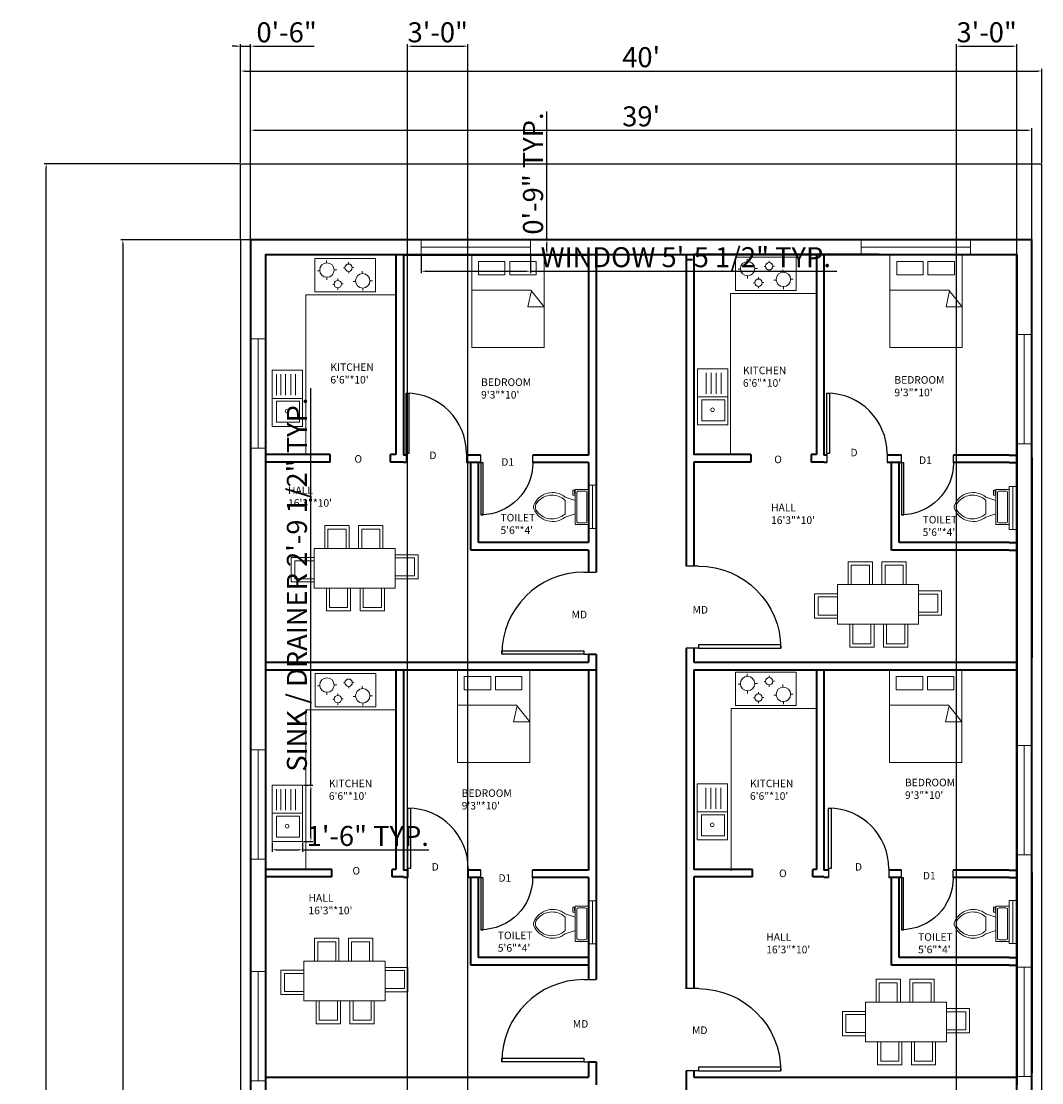
# Model space of a CAD drawing. Units: inches. Extents: x 1947 to 2903, y 1974 to 3472.
# Tile 5 of 5: x 2132 to 2743, y 2836 to 3472. Entities that reach past the tile are written whole.
import ezdxf

# ---------------------------------------------------------------- set-up
doc = ezdxf.new("R2010")
doc.units = ezdxf.units.IN
for name, color, linetype, lineweight in [('A-ANNO-DIMS', 2, 'Continuous', 18), ('A-ANNO-TEXT', 7, 'Continuous', 18), ('A-AREA-IDEN', 7, 'Continuous', 18), ('A-DOOR', 3, 'Continuous', 25), ('A-EQPM', 8, 'Continuous', 18), ('A-FLOR-CASE', 8, 'Continuous', 18), ('A-FLOR-FIXT', 9, 'Continuous', 18), ('A-FURN', 8, 'Continuous', 18), ('A-GLAZ', 4, 'Continuous', 18), ('A-GLAZ-VENT', 4, 'Continuous', 18), ('A-WALL', 7, 'Continuous', 35), ('C-PROP', 1, 'Continuous', 25)]:
    doc.layers.add(name, color=color, linetype=linetype, lineweight=lineweight)
doc.styles.get("Standard").update_dxf_attribs({"font": 'arial.ttf'})
doc.dimstyles.new('ISO-25', dxfattribs={"dimtxt": 12, "dimasz": 2.5, "dimexe": 1.25, "dimexo": 0.625, "dimtad": 1, "dimdec": 0, "dimlunit": 4, "dimtxsty": 'Standard', "dimcen": 2.5, "dimadec": 0, "dimazin": 0, "dimtfac": 1, "dimtdec": 0, "dimtmove": 0, "dimatfit": 3, "dimfxl": 1, "dimarcsym": 0})

# ---------------------------------------------------------------- blocks, each defined once
blk = doc.blocks.new('*U2')
for p, q in [((0, 0), (0, -6)), ((40, 0), (40, -6))]:
    blk.add_line(p, q)
blk.add_lwpolyline([(0, 0), (0, 40), (1.75, 40), (1.75, 0)], close=True)
blk.add_arc((0, 0), 40, 0, 90)
blk = doc.blocks.new('*U4')
for p, q in [((9.5, -6), (9.5, -2)), ((-10, -8.5), (-8, -8.5)), ((-10, -9.5), (-10, -8.5)), ((-7, -9.5), (-10, -9.5)), ((-8, -8.5), (-8, -8)), ((-7, -8), (-7, -9.5)), ((-4, -8), (-6, -14)), ((4, -8), (6, -14)), ((4, -14), (-4, -14))]:
    blk.add_line(p, q)
blk.add_lwpolyline([(10.5, -8), (10.5, 0), (-10.5, 0), (-10.5, -8)], close=True)
for points in [[(-9.5, -2), (-9.5, -6)], [(8.5, -1), (-8.5, -1)], [(-8.5, -7), (8.5, -7)]]:
    blk.add_lwpolyline(points)
for centre, radius, start, end in [((-8.62, -1.88), 0.884, 81.8699, 188.1301), ((-8.62, -6.12), 0.884, 171.8699, 278.1301), ((8.62, -1.88), 0.884, 351.8699, 98.1301), ((8.62, -6.12), 0.884, 261.8699, 8.1301), ((3.52, -21.58), 12.17, 141.46911, 247.97143), ((4.2, -21.82), 11.33, 136.36773, 238.94682), ((-3.52, -21.58), 12.17, 292.02843, 38.53071), ((-4.2, -21.82), 11.33, 301.05301, 43.63209), ((0, -27.88), 4, 245.73182, 294.26817), ((0, -29), 4, 254.86053, 285.13947)]:
    blk.add_arc(centre, radius, start, end)
blk = doc.blocks.new('*D5')
at = {"layer": 'A-ANNO-DIMS', "color": 0, "lineweight": -2, "transparency": 16777216}
for p, q in [((2269.11, 3342.03), (2269.11, 3408.29)), ((2271.61, 3407.04), (2734.61, 3407.04)), ((2737.11, 3342.03), (2737.11, 3408.29))]:
    blk.add_line(p, q, dxfattribs=at)
at = {"layer": 'A-ANNO-DIMS', "color": 0, "lineweight": 100, "transparency": 16777216}
for points in [[(2271.61, 3407.46), (2271.61, 3406.63), (2269.11, 3407.04)], [(2734.61, 3407.46), (2734.61, 3406.63), (2737.11, 3407.04)]]:
    blk.add_solid(points, dxfattribs=at)
at = {"layer": 'Defpoints', "color": 0, "lineweight": 100, "transparency": 16777216}
for p in [(2737.11, 3407.04), (2269.11, 3341.41), (2737.11, 3341.41)]:
    blk.add_point(p, dxfattribs=at)
at = {"layer": 'A-ANNO-DIMS', "color": 0, "transparency": 16777216, "insert": (2503.11, 3413.8), "char_height": 12, "attachment_point": 5}
blk.add_mtext("39'", dxfattribs=at)
blk = doc.blocks.new('*D6')
at = {"layer": 'A-ANNO-DIMS', "color": 0, "lineweight": -2, "transparency": 16777216}
for p, q in [((2268.49, 3341.41), (2191.31, 3341.41)), ((2192.56, 3338.91), (2192.56, 2230.91)), ((2268.49, 2228.41), (2191.31, 2228.41))]:
    blk.add_line(p, q, dxfattribs=at)
at = {"layer": 'A-ANNO-DIMS', "color": 0, "lineweight": 100, "transparency": 16777216}
for points in [[(2192.15, 3338.91), (2192.98, 3338.91), (2192.56, 3341.41)], [(2192.15, 2230.91), (2192.98, 2230.91), (2192.56, 2228.41)]]:
    blk.add_solid(points, dxfattribs=at)
at = {"layer": 'Defpoints', "color": 0, "lineweight": 100, "transparency": 16777216}
for p in [(2269.11, 3341.41), (2192.56, 2228.41), (2269.11, 2228.41)]:
    blk.add_point(p, dxfattribs=at)
at = {"layer": 'A-ANNO-DIMS', "color": 0, "transparency": 16777216, "insert": (2185.81, 2784.91), "char_height": 12, "attachment_point": 5, "rotation": 90}
blk.add_mtext('92\'-9"', dxfattribs=at)
blk = doc.blocks.new('*D7')
at = {"layer": 'A-ANNO-DIMS', "color": 0, "lineweight": -2, "transparency": 16777216}
for p, q in [((2263.11, 3387.59), (2263.11, 3443.75)), ((2265.61, 3442.5), (2740.61, 3442.5)), ((2743.11, 3387.59), (2743.11, 3443.75))]:
    blk.add_line(p, q, dxfattribs=at)
at = {"layer": 'A-ANNO-DIMS', "color": 0, "lineweight": 100, "transparency": 16777216}
for points in [[(2265.61, 3442.92), (2265.61, 3442.09), (2263.11, 3442.5)], [(2740.61, 3442.92), (2740.61, 3442.09), (2743.11, 3442.5)]]:
    blk.add_solid(points, dxfattribs=at)
at = {"layer": 'Defpoints', "color": 0, "lineweight": 100, "transparency": 16777216}
for p in [(2743.11, 3442.5), (2263.11, 3386.97), (2743.11, 3386.97)]:
    blk.add_point(p, dxfattribs=at)
at = {"layer": 'A-ANNO-DIMS', "color": 0, "transparency": 16777216, "insert": (2503.11, 3449.26), "char_height": 12, "attachment_point": 5}
blk.add_mtext("40'", dxfattribs=at)
blk = doc.blocks.new('*D8')
at = {"layer": 'A-ANNO-DIMS', "color": 0, "lineweight": -2, "transparency": 16777216}
for p, q in [((2262.49, 3386.97), (2145.36, 3386.97)), ((2146.61, 2187.91), (2146.61, 3384.47)), ((2262.49, 2185.41), (2145.36, 2185.41))]:
    blk.add_line(p, q, dxfattribs=at)
at = {"layer": 'A-ANNO-DIMS', "color": 0, "lineweight": 100, "transparency": 16777216}
for points in [[(2146.19, 3384.47), (2147.03, 3384.47), (2146.61, 3386.97)], [(2146.19, 2187.91), (2147.03, 2187.91), (2146.61, 2185.41)]]:
    blk.add_solid(points, dxfattribs=at)
at = {"layer": 'Defpoints', "color": 0, "lineweight": 100, "transparency": 16777216}
for p in [(2146.61, 3386.97), (2263.11, 3386.97), (2263.11, 2185.41)]:
    blk.add_point(p, dxfattribs=at)
at = {"layer": 'A-ANNO-DIMS', "color": 0, "transparency": 16777216, "insert": (2139.86, 2786.19), "char_height": 12, "attachment_point": 5, "rotation": 90}
blk.add_mtext('100\'-2"', dxfattribs=at)
blk = doc.blocks.new('BED-TWO-PILLOWS')
for p, q in [((0, 34.29), (35.37, 34.29)), ((33.59, 24.29), (35.7, 33.87)), ((35.37, 34.29), (43.32, 24.29)), ((43.32, 24.29), (33.59, 24.29))]:
    blk.add_line(p, q)
for points in [[(0, 55.57), (43.32, 55.57), (43.32, 0), (0, 0)], [(4.07, 51.54), (19.88, 51.54), (19.88, 43.48), (4.07, 43.48)], [(22.78, 51.54), (38.59, 51.54), (38.59, 43.48), (22.78, 43.48)]]:
    blk.add_lwpolyline(points, close=True)
blk = doc.blocks.new('DINING-SET-6')
for p, q in [((20.16, 37.5), (20.16, 51.24)), ((20.16, 51.24), (34.7, 51.24)), ((34.7, 51.24), (34.7, 37.5)), ((40.4, 37.5), (40.4, 51.24)), ((40.4, 51.24), (54.94, 51.24)), ((54.94, 51.24), (54.94, 37.5)), ((13.74, 31.99), (0, 31.99)), ((0, 31.99), (0, 17.45)), ((62.33, 33.71), (76.07, 33.71)), ((76.07, 33.71), (76.07, 19.17)), ((76.07, 19.17), (62.33, 19.17)), ((0, 17.45), (13.74, 17.45)), ((21.08, 13.74), (21.08, 0)), ((35.62, 0), (35.62, 13.74)), ((41.32, 13.74), (41.32, 0)), ((55.86, 0), (55.86, 13.74)), ((21.08, 0), (35.62, 0)), ((41.32, 0), (55.86, 0))]:
    blk.add_line(p, q)
for points in [[(22.02, 37.5), (32.87, 37.5), (32.87, 49.12), (22.02, 49.12)], [(42.26, 37.5), (53.11, 37.5), (53.11, 49.12), (42.26, 49.12)], [(13.74, 13.74), (62.33, 13.74), (62.33, 37.5), (13.74, 37.5)], [(62.33, 31.85), (62.33, 21), (73.95, 21), (73.95, 31.85)], [(13.74, 30.13), (13.74, 19.28), (2.12, 19.28), (2.12, 30.13)], [(22.94, 13.74), (33.79, 13.74), (33.79, 2.12), (22.94, 2.12)], [(43.18, 13.74), (54.03, 13.74), (54.03, 2.12), (43.18, 2.12)]]:
    blk.add_lwpolyline(points, close=True)
blk = doc.blocks.new('COOKTOP-4-BURNER')
for p, q in [((6.9, 17.32), (6.9, 18.83)), ((11.47, 13.09), (13.05, 13.09)), ((17.95, 14.27), (17.07, 14.27)), ((20.11, 16.62), (20.11, 17.76)), ((22.35, 14.5), (23.33, 14.5)), ((2.85, 12.63), (1.48, 12.63)), ((7.15, 8.69), (7.15, 7.15)), ((13.68, 6.8), (13.68, 7.94)), ((20.18, 12.22), (20.18, 11.07)), ((28.35, 10.88), (28.35, 12.39)), ((32.92, 6.64), (34.51, 6.64)), ((11.52, 4.44), (10.65, 4.44)), ((13.75, 2.39), (13.75, 1.25)), ((15.92, 4.68), (16.91, 4.68)), ((24.3, 6.18), (22.93, 6.18)), ((28.6, 2.24), (28.6, 0.7))]:
    blk.add_line(p, q)
blk.add_lwpolyline([(0, 0), (36.35, 0), (36.35, 19.93), (0, 19.93)], close=True)
for centre, radius in [((7.15, 13.01), 4.32), ((20.14, 14.42), 2.2), ((13.72, 4.6), 2.2), ((28.6, 6.56), 4.32)]:
    blk.add_circle(centre, radius)
blk = doc.blocks.new('SINK-DRAINER-5')
for p, q in [((2.58, 18.66), (2.58, 31.31)), ((5.19, 18.66), (5.19, 31.31)), ((8.1, 18.66), (8.1, 31.31)), ((11.22, 18.66), (11.22, 31.31)), ((14.13, 18.66), (14.13, 31.31)), ((0, 16.81), (18.23, 16.81))]:
    blk.add_line(p, q)
for points in [[(0, 0), (18.23, 0), (18.23, 33.61), (0, 33.61)], [(2.68, 15.14), (16.44, 15.14), (16.44, 2.49), (2.68, 2.49)]]:
    blk.add_lwpolyline(points, close=True)
blk.add_circle((9.01, 9.12), 1.11)
blk = doc.blocks.new('SINK-DRAINER-4')
for p, q in [((5.19, 18.66), (5.19, 31.31)), ((8.1, 18.66), (8.1, 31.31)), ((11.22, 18.66), (11.22, 31.31)), ((14.13, 18.66), (14.13, 31.31)), ((0, 16.81), (18.23, 16.81))]:
    blk.add_line(p, q)
for points in [[(0, 0), (18.23, 0), (18.23, 33.61), (0, 33.61)], [(2.68, 15.14), (16.44, 15.14), (16.44, 2.49), (2.68, 2.49)]]:
    blk.add_lwpolyline(points, close=True)
blk.add_circle((9.01, 9.12), 1.11)
blk = doc.blocks.new('WINDOW-EXTERIOR')
blk.add_line((0, 4.5), (65.51, 4.5))
blk.add_lwpolyline([(0, 0), (65.51, 0), (65.51, 9), (0, 9)], close=True)
blk = doc.blocks.new('VENT-TOILET')
blk.add_line((2.25, 0), (2.25, 25.89))
blk.add_lwpolyline([(0, 25.89), (4.5, 25.89), (4.5, 0), (0, 0)], close=True)
blk = doc.blocks.new('COOKTOP-4-BURNER-B')
for p, q in [((11.47, 13.09), (13.05, 13.09)), ((17.95, 14.27), (17.07, 14.27)), ((22.35, 14.5), (23.33, 14.5)), ((2.85, 12.63), (1.48, 12.63)), ((7.15, 8.69), (7.15, 7.15)), ((13.68, 6.8), (13.68, 7.94)), ((20.18, 12.22), (20.18, 11.07)), ((28.35, 10.88), (28.35, 12.39)), ((32.92, 6.64), (34.51, 6.64)), ((11.52, 4.44), (10.65, 4.44)), ((13.75, 2.4), (13.75, 1.25)), ((15.92, 4.68), (16.91, 4.68)), ((24.3, 6.18), (22.93, 6.18)), ((28.6, 2.24), (28.6, 0.71))]:
    blk.add_line(p, q)
blk.add_lwpolyline([(0, 0), (36.35, 0), (36.35, 19.93), (0, 19.93)], close=True)
for centre, radius in [((7.15, 13.01), 4.32), ((20.14, 14.42), 2.2), ((13.72, 4.6), 2.2), ((28.6, 6.56), 4.32)]:
    blk.add_circle(centre, radius)
blk = doc.blocks.new('*D17')
at = {"layer": 'A-ANNO-DIMS', "color": 0, "lineweight": -2, "transparency": 16777216}
for p, q in [((2371.28, 3331.78), (2371.28, 3321.33)), ((2436.79, 3331.78), (2436.79, 3321.33)), ((2373.78, 3322.58), (2434.29, 3322.58)), ((2436.79, 3322.58), (2620.35, 3322.58))]:
    blk.add_line(p, q, dxfattribs=at)
at = {"layer": 'A-ANNO-DIMS', "color": 0, "lineweight": 100, "transparency": 16777216}
for points in [[(2373.78, 3323), (2373.78, 3322.16), (2371.28, 3322.58)], [(2434.29, 3323), (2434.29, 3322.16), (2436.79, 3322.58)]]:
    blk.add_solid(points, dxfattribs=at)
at = {"layer": 'Defpoints', "color": 0, "lineweight": 100, "transparency": 16777216}
for p in [(2371.28, 3332.41), (2436.79, 3332.41), (2436.79, 3322.58)]:
    blk.add_point(p, dxfattribs=at)
at = {"layer": 'A-ANNO-DIMS', "color": 0, "transparency": 16777216, "insert": (2529.82, 3329.41), "char_height": 12, "attachment_point": 5}
blk.add_mtext('WINDOW 5\'-5 1/2" TYP.', dxfattribs=at)
blk = doc.blocks.new('*D18')
at = {"layer": 'A-ANNO-DIMS', "color": 0, "lineweight": -2, "transparency": 16777216}
for p, q in [((2446.62, 3341.41), (2446.62, 3418.3)), ((2437.42, 3341.41), (2447.87, 3341.41)), ((2446.62, 3334.91), (2446.62, 3338.91)), ((2437.42, 3332.41), (2447.87, 3332.41))]:
    blk.add_line(p, q, dxfattribs=at)
at = {"layer": 'A-ANNO-DIMS', "color": 0, "lineweight": 100, "transparency": 16777216}
for points in [[(2446.2, 3338.91), (2447.03, 3338.91), (2446.62, 3341.41)], [(2446.2, 3334.91), (2447.03, 3334.91), (2446.62, 3332.41)]]:
    blk.add_solid(points, dxfattribs=at)
at = {"layer": 'Defpoints', "color": 0, "lineweight": 100, "transparency": 16777216}
for p in [(2436.79, 3341.41), (2446.62, 3341.41), (2436.79, 3332.41)]:
    blk.add_point(p, dxfattribs=at)
at = {"layer": 'A-ANNO-DIMS', "color": 0, "transparency": 16777216, "insert": (2439.86, 3381.1), "char_height": 12, "attachment_point": 5, "rotation": 90}
blk.add_mtext('0\'-9" TYP.', dxfattribs=at)
blk = doc.blocks.new('*D27')
at = {"layer": 'A-ANNO-DIMS', "color": 0, "lineweight": -2, "transparency": 16777216}
for p, q in [((2305.22, 3014.51), (2305.22, 3252.52)), ((2300.8, 3014.51), (2306.47, 3014.51)), ((2305.22, 2983.4), (2305.22, 3012.01)), ((2300.8, 2980.9), (2306.47, 2980.9))]:
    blk.add_line(p, q, dxfattribs=at)
at = {"layer": 'A-ANNO-DIMS', "color": 0, "lineweight": 100, "transparency": 16777216}
for points in [[(2304.8, 3012.01), (2305.64, 3012.01), (2305.22, 3014.51)], [(2304.8, 2983.4), (2305.64, 2983.4), (2305.22, 2980.9)]]:
    blk.add_solid(points, dxfattribs=at)
at = {"layer": 'Defpoints', "color": 0, "lineweight": 100, "transparency": 16777216}
for p in [(2300.18, 3014.51), (2305.22, 3014.51), (2300.18, 2980.9)]:
    blk.add_point(p, dxfattribs=at)
at = {"layer": 'A-ANNO-DIMS', "color": 0, "transparency": 16777216, "insert": (2298.39, 3134.77), "char_height": 12, "attachment_point": 5, "rotation": 90}
blk.add_mtext('SINK / DRAINER 2\'-9 1/2" TYP.', dxfattribs=at)
blk = doc.blocks.new('*D28')
at = {"layer": 'A-ANNO-DIMS', "color": 0, "lineweight": -2, "transparency": 16777216}
for p, q in [((2281.94, 2980.27), (2281.94, 2974.61)), ((2300.18, 2980.27), (2300.18, 2974.61)), ((2284.44, 2975.86), (2297.68, 2975.86)), ((2300.18, 2975.86), (2375.94, 2975.86))]:
    blk.add_line(p, q, dxfattribs=at)
at = {"layer": 'A-ANNO-DIMS', "color": 0, "lineweight": 100, "transparency": 16777216}
for points in [[(2284.44, 2976.27), (2284.44, 2975.44), (2281.94, 2975.86)], [(2297.68, 2976.27), (2297.68, 2975.44), (2300.18, 2975.86)]]:
    blk.add_solid(points, dxfattribs=at)
at = {"layer": 'Defpoints', "color": 0, "lineweight": 100, "transparency": 16777216}
for p in [(2281.94, 2980.9), (2300.18, 2980.9), (2300.18, 2975.86)]:
    blk.add_point(p, dxfattribs=at)
at = {"layer": 'A-ANNO-DIMS', "color": 0, "transparency": 16777216, "insert": (2339.31, 2982.61), "char_height": 12, "attachment_point": 5}
blk.add_mtext('1\'-6" TYP.', dxfattribs=at)
blk = doc.blocks.new('*D36')
at = {"layer": 'A-ANNO-DIMS', "color": 0, "lineweight": -2, "transparency": 16777216}
for p, q in [((2692.11, 2238.03), (2692.11, 3458.67)), ((2694.61, 3457.42), (2725.61, 3457.42)), ((2728.11, 2238.03), (2728.11, 3458.67))]:
    blk.add_line(p, q, dxfattribs=at)
at = {"layer": 'A-ANNO-DIMS', "color": 0, "lineweight": 100, "transparency": 16777216}
for points in [[(2694.61, 3457.83), (2694.61, 3457), (2692.11, 3457.42)], [(2725.61, 3457.83), (2725.61, 3457), (2728.11, 3457.42)]]:
    blk.add_solid(points, dxfattribs=at)
at = {"layer": 'Defpoints', "color": 0, "lineweight": 100, "transparency": 16777216}
for p in [(2728.11, 3457.42), (2692.11, 2237.41), (2728.11, 2237.41)]:
    blk.add_point(p, dxfattribs=at)
at = {"layer": 'A-ANNO-DIMS', "color": 0, "transparency": 16777216, "insert": (2710.11, 3464.17), "char_height": 12, "attachment_point": 5}
blk.add_mtext('3\'-0"', dxfattribs=at)
blk = doc.blocks.new('*D40')
at = {"layer": 'A-ANNO-DIMS', "color": 0, "lineweight": -2, "transparency": 16777216}
for p, q in [((2363.18, 2467.02), (2363.18, 3458.67)), ((2365.68, 3457.42), (2396.82, 3457.42)), ((2399.32, 2467.02), (2399.32, 3458.67))]:
    blk.add_line(p, q, dxfattribs=at)
at = {"layer": 'A-ANNO-DIMS', "color": 0, "lineweight": 100, "transparency": 16777216}
for points in [[(2365.68, 3457.83), (2365.68, 3457), (2363.18, 3457.42)], [(2396.82, 3457.83), (2396.82, 3457), (2399.32, 3457.42)]]:
    blk.add_solid(points, dxfattribs=at)
at = {"layer": 'Defpoints', "color": 0, "lineweight": 100, "transparency": 16777216}
for p in [(2399.32, 3457.42), (2363.18, 2466.39), (2399.32, 2466.39)]:
    blk.add_point(p, dxfattribs=at)
at = {"layer": 'A-ANNO-DIMS', "color": 0, "transparency": 16777216, "insert": (2381.25, 3464.17), "char_height": 12, "attachment_point": 5}
blk.add_mtext('3\'-0"', dxfattribs=at)
blk = doc.blocks.new('*D43')
at = {"layer": 'A-ANNO-DIMS', "color": 0, "lineweight": -2, "transparency": 16777216}
for p, q in [((2260.61, 3457.42), (2258.11, 3457.42)), ((2263.11, 3387.59), (2263.11, 3458.67)), ((2263.11, 3457.42), (2269.11, 3457.42)), ((2269.11, 3342.03), (2269.11, 3458.67)), ((2271.61, 3457.42), (2307.26, 3457.42))]:
    blk.add_line(p, q, dxfattribs=at)
at = {"layer": 'A-ANNO-DIMS', "color": 0, "lineweight": 100, "transparency": 16777216}
for points in [[(2260.61, 3457.83), (2260.61, 3457), (2263.11, 3457.42)], [(2271.61, 3457.83), (2271.61, 3457), (2269.11, 3457.42)]]:
    blk.add_solid(points, dxfattribs=at)
at = {"layer": 'Defpoints', "color": 0, "lineweight": 100, "transparency": 16777216}
for p in [(2269.11, 3457.42), (2263.11, 3386.97), (2269.11, 3341.41)]:
    blk.add_point(p, dxfattribs=at)
at = {"layer": 'A-ANNO-DIMS', "color": 0, "transparency": 16777216, "insert": (2290.68, 3464.17), "char_height": 12, "attachment_point": 5}
blk.add_mtext('0\'-6"', dxfattribs=at)

msp = doc.modelspace()

# ---------------------------------------------------------------- linework, layer by layer
at = {"layer": 'A-FLOR-CASE'}
for p, q in [((2356.11, 3332.41), (2356.11, 3308.41)), ((2302.11, 3212.73), (2302.11, 3308.41)), ((2356.11, 3308.41), (2302.11, 3308.41)), ((2556.71, 3213.57), (2556.71, 3309.24)), ((2608.11, 3309.24), (2556.71, 3309.24)), ((2278.11, 3212.73), (2302.11, 3212.73)), ((2302.11, 2964.06), (2302.11, 3059.73)), ((2356.11, 3059.73), (2302.11, 3059.73)), ((2557.05, 2963.31), (2557.05, 3060.58)), ((2608.11, 3060.58), (2557.05, 3060.58)), ((2278.11, 2964.06), (2302.11, 2964.06))]:
    msp.add_line(p, q, dxfattribs=at)
at = {"layer": 'A-WALL'}
for p, q in [((2356.11, 3332.41), (2356.11, 3212.73)), ((2360.61, 3332.41), (2360.61, 3212.41)), ((2360.61, 3332.41), (2471.61, 3332.41)), ((2471.61, 3332.41), (2471.61, 3212.41)), ((2476.11, 3332.41), (2476.11, 3207.91)), ((2530.11, 3332.6), (2530.11, 3208.1)), ((2645.61, 3332.6), (2534.61, 3332.6)), ((2534.61, 3332.6), (2534.61, 3212.6)), ((2608.11, 3332.41), (2608.11, 3212.73)), ((2612.61, 3332.41), (2612.61, 3212.41)), ((2728.11, 3332.41), (2728.11, 3207.91)), ((2316.73, 3212.73), (2278.11, 3212.73)), ((2316.73, 3208.23), (2316.73, 3212.73)), ((2356.11, 3212.73), (2352.86, 3212.73)), ((2352.86, 3208.23), (2352.86, 3212.73)), ((2362.29, 3212.41), (2360.61, 3212.41)), ((2407.08, 3212.41), (2398.43, 3212.41)), ((2471.61, 3212.41), (2438.18, 3212.41)), ((2530.11, 3212.73), (2530.11, 3212.73)), ((2568.73, 3212.73), (2534.61, 3212.73)), ((2568.73, 3212.73), (2568.73, 3208.23)), ((2608.11, 3212.73), (2604.86, 3212.73)), ((2604.86, 3212.73), (2604.86, 3208.23)), ((2614.29, 3212.41), (2612.61, 3212.41)), ((2659.08, 3212.41), (2650.43, 3212.41)), ((2723.61, 3212.41), (2690.18, 3212.41)), ((2723.61, 3212.41), (2728.11, 3212.41)), ((2278.11, 3208.23), (2278.11, 3088.23)), ((2316.73, 3208.23), (2278.11, 3208.23)), ((2360.61, 3208.23), (2352.86, 3208.23)), ((2362.29, 3207.91), (2360.61, 3207.91)), ((2407.08, 3207.91), (2398.43, 3207.91)), ((2401.11, 3155.41), (2401.11, 3207.91)), ((2405.61, 3159.91), (2405.61, 3207.91)), ((2471.61, 3207.91), (2438.18, 3207.91)), ((2471.61, 3207.91), (2471.61, 3159.91)), ((2476.11, 3207.91), (2476.11, 3142.22)), ((2530.11, 3208.23), (2530.11, 3208.23)), ((2530.11, 3208.1), (2530.11, 3145.81)), ((2568.73, 3208.23), (2534.61, 3208.23)), ((2534.61, 3208.23), (2534.61, 3145.81)), ((2612.61, 3208.23), (2604.86, 3208.23)), ((2614.29, 3207.91), (2612.61, 3207.91)), ((2659.08, 3207.91), (2650.43, 3207.91)), ((2653.11, 3155.41), (2653.11, 3207.91)), ((2657.61, 3159.91), (2657.61, 3207.91)), ((2723.61, 3207.91), (2690.18, 3207.91)), ((2723.61, 3207.91), (2728.11, 3207.91)), ((2728.11, 3208.43), (2728.11, 3088.43)), ((2728.11, 3207.91), (2728.11, 3142.22)), ((2737.11, 3210.89), (2737.11, 3090.89)), ((2471.61, 3155.41), (2401.11, 3155.41)), ((2471.61, 3159.91), (2405.61, 3159.91)), ((2471.61, 3155.41), (2471.61, 3142.22)), ((2723.61, 3155.41), (2653.11, 3155.41)), ((2723.61, 3159.91), (2657.61, 3159.91)), ((2723.61, 3159.91), (2728.11, 3159.91)), ((2723.61, 3155.41), (2728.11, 3155.41)), ((2471.61, 3093.01), (2476.11, 3093.01)), ((2471.61, 3093.01), (2471.61, 3088.23)), ((2476.11, 3093.01), (2476.11, 3083.73)), ((2530.11, 3096.61), (2530.11, 2892.64)), ((2534.61, 3096.61), (2534.61, 3088.23)), ((2728.11, 3093.01), (2728.11, 3083.73)), ((2278.11, 3088.23), (2471.61, 3088.23)), ((2534.61, 3088.23), (2723.61, 3088.23)), ((2723.61, 3088.23), (2728.11, 3088.23)), ((2278.11, 3083.73), (2476.11, 3083.73)), ((2356.11, 3083.73), (2356.11, 2964.06)), ((2360.61, 3083.73), (2360.61, 2963.73)), ((2360.61, 3083.73), (2471.61, 3083.73)), ((2471.61, 3083.73), (2471.61, 2963.73)), ((2476.11, 3083.73), (2476.11, 2959.23)), ((2534.61, 3083.73), (2728.11, 3083.73)), ((2534.61, 3083.73), (2534.61, 2964.06)), ((2608.11, 3083.73), (2608.11, 2964.06)), ((2612.61, 3083.73), (2612.61, 2963.73)), ((2612.61, 3083.73), (2723.61, 3083.73)), ((2728.11, 3083.73), (2728.11, 2959.23)), ((2317.8, 2964.06), (2278.11, 2964.06)), ((2316.73, 2964.06), (2278.11, 2964.06)), ((2278.11, 2959.56), (2278.11, 2839.56)), ((2317.8, 2959.56), (2278.11, 2959.56)), ((2317.8, 2959.56), (2317.8, 2964.06)), ((2356.11, 2964.06), (2353.94, 2964.06)), ((2353.94, 2959.56), (2353.94, 2964.06)), ((2360.61, 2959.56), (2353.94, 2959.56)), ((2363.37, 2963.73), (2360.61, 2963.73)), ((2363.37, 2959.23), (2360.61, 2959.23)), ((2406.98, 2963.73), (2399.51, 2963.73)), ((2406.98, 2959.23), (2399.51, 2959.23)), ((2401.11, 2906.73), (2401.11, 2959.23)), ((2405.61, 2911.23), (2405.61, 2959.23)), ((2471.61, 2963.73), (2438.08, 2963.73)), ((2471.61, 2959.23), (2438.08, 2959.23)), ((2471.61, 2959.23), (2471.61, 2911.23)), ((2476.11, 2959.23), (2476.11, 2898.05)), ((2530.11, 2964.06), (2530.11, 2964.06)), ((2530.11, 2959.56), (2530.11, 2959.56)), ((2569.81, 2964.06), (2534.61, 2964.06)), ((2569.81, 2959.56), (2534.61, 2959.56)), ((2534.61, 2959.56), (2534.61, 2892.64)), ((2569.81, 2959.56), (2569.81, 2964.06)), ((2608.11, 2964.06), (2605.94, 2964.06)), ((2605.94, 2959.56), (2605.94, 2964.06)), ((2612.61, 2959.56), (2605.94, 2959.56)), ((2615.37, 2963.73), (2612.61, 2963.73)), ((2615.37, 2959.23), (2612.61, 2959.23)), ((2658.98, 2963.73), (2651.51, 2963.73)), ((2658.98, 2959.23), (2651.51, 2959.23)), ((2653.11, 2906.73), (2653.11, 2959.23)), ((2657.61, 2911.23), (2657.61, 2959.23)), ((2723.61, 2963.73), (2690.08, 2963.73)), ((2723.61, 2959.23), (2690.08, 2959.23)), ((2723.61, 2963.73), (2728.11, 2963.73)), ((2723.61, 2959.23), (2728.11, 2959.23)), ((2728.11, 2959.76), (2728.11, 2839.76)), ((2728.11, 2959.23), (2728.11, 2898.05)), ((2737.11, 2962.22), (2737.11, 2842.22)), ((2471.61, 2911.23), (2405.61, 2911.23)), ((2471.61, 2911.23), (2471.61, 2898.05)), ((2723.61, 2911.23), (2657.61, 2911.23)), ((2723.61, 2911.23), (2728.11, 2911.23)), ((2471.61, 2906.73), (2401.11, 2906.73)), ((2471.61, 2906.73), (2471.61, 2898.05)), ((2723.61, 2906.73), (2653.11, 2906.73)), ((2723.61, 2906.73), (2728.11, 2906.73)), ((2471.61, 2848.84), (2471.61, 2844.06)), ((2471.61, 2848.84), (2476.11, 2848.84)), ((2471.61, 2848.84), (2471.61, 2839.56)), ((2476.11, 2848.84), (2476.11, 2839.56)), ((2476.11, 2848.84), (2476.11, 2835.06)), ((2530.11, 2843.44), (2530.11, 2643.97)), ((2534.61, 2843.44), (2534.61, 2839.56)), ((2728.11, 2848.84), (2728.11, 2835.06)), ((2728.11, 2848.84), (2728.11, 2839.56)), ((2278.11, 2839.56), (2471.61, 2839.56)), ((2278.11, 2839.56), (2471.61, 2839.56)), ((2534.61, 2839.56), (2723.61, 2839.56)), ((2534.61, 2839.56), (2723.61, 2839.56)), ((2723.61, 2839.56), (2728.11, 2839.56))]:
    msp.add_line(p, q, dxfattribs=at)
for points in [[(2269.11, 2228.41), (2737.11, 2228.41), (2737.11, 3341.41), (2269.11, 3341.41)], [(2278.11, 2237.41), (2728.11, 2237.41), (2728.11, 3332.41), (2278.11, 3332.41)]]:
    msp.add_lwpolyline(points, close=True, dxfattribs=at)
at = {"layer": 'C-PROP'}
for p, q in [((2263.11, 3341.17), (2263.11, 3386.97)), ((2263.11, 3386.97), (2743.11, 3386.97)), ((2743.11, 3341.41), (2743.11, 3386.97)), ((2263.11, 3341.41), (2263.11, 2228.41)), ((2743.11, 2228.41), (2743.11, 3341.41))]:
    msp.add_line(p, q, dxfattribs=at)

# ---------------------------------------------------------------- block references
at = {"layer": 'A-DOOR', "xscale": 0.9034599273514711, "yscale": 0.9034599273514711, "zscale": 0.9034599273514711}
for p in [(2362.29, 3213.33), (2614.29, 3213.33), (2363.37, 2964.65), (2615.37, 2964.65)]:
    msp.add_blockref('*U2', p, dxfattribs=at)
at = {"layer": 'A-DOOR'}
for p, xscale, yscale, zscale, rotation in [((2407.08, 3207.74), -0.7774936004188162, 0.7774936004188162, 0.7774936004188162, 180), ((2659.08, 3207.74), -0.7774936004188162, 0.7774936004188162, 0.7774936004188162, 180), ((2537.49, 3096.61), -1.23010588698369, 1.23010588698369, 1.23010588698369, 270), ((2468.73, 3093.01), 1.23010588698369, 1.23010588698369, 1.23010588698369, 90.00000000000003), ((2406.98, 2959.07), -0.7774936004188162, 0.7774936004188162, 0.7774936004188162, 180), ((2658.98, 2959.07), -0.7774936004188162, 0.7774936004188162, 0.7774936004188162, 180), ((2468.73, 2848.84), 1.23010588698369, 1.23010588698369, 1.23010588698369, 90.00000000000003), ((2537.49, 2843.44), -1.23010588698369, 1.23010588698369, 1.23010588698369, 270)]:
    msp.add_blockref('*U2', p, dxfattribs=dict(at, xscale=xscale, yscale=yscale, zscale=zscale, rotation=rotation))
at = {"layer": 'A-EQPM'}
for name, p in [('COOKTOP-4-BURNER', (2307.68, 3310.24)), ('COOKTOP-4-BURNER', (2559.69, 3311.08)), ('COOKTOP-4-BURNER-B', (2307.69, 3061.57)), ('COOKTOP-4-BURNER', (2559.69, 3062.42))]:
    msp.add_blockref(name, p, dxfattribs=at)
at = {"layer": 'A-FLOR-FIXT'}
for name, p in [('SINK-DRAINER-5', (2281.94, 3229.57)), ('SINK-DRAINER-4', (2536.86, 3230.41)), ('SINK-DRAINER-4', (2536.66, 2981.74)), ('SINK-DRAINER-5', (2281.94, 2980.9))]:
    msp.add_blockref(name, p, dxfattribs=at)
at = {"layer": 'A-FLOR-FIXT', "rotation": 270}
for p in [(2471.61, 3181.26), (2723.61, 3181.26), (2471.61, 2931.5), (2723.61, 2931.5)]:
    msp.add_blockref('*U4', p, dxfattribs=at)
at = {"layer": 'A-FURN'}
for name, p in [('BED-TWO-PILLOWS', (2401.61, 3276.84)), ('BED-TWO-PILLOWS', (2652.15, 3276.84)), ('DINING-SET-6', (2293.42, 3118.96)), ('DINING-SET-6', (2606.98, 3097.23)), ('BED-TWO-PILLOWS', (2393.06, 3028.17)), ('BED-TWO-PILLOWS', (2651.9, 3028.17)), ('DINING-SET-6', (2287.3, 2871.67)), ('DINING-SET-6', (2623.68, 2847))]:
    msp.add_blockref(name, p, dxfattribs=at)
at = {"layer": 'A-GLAZ'}
for p in [(2371.28, 3332.41), (2634.89, 3332.41)]:
    msp.add_blockref('WINDOW-EXTERIOR', p, dxfattribs=at)
for p, rotation in [((2728.11, 3284.72), 269.9999999999986), ((2269.11, 3282.06), 269.9999999999993), ((2269.11, 3035.72), 269.9999999999993), ((2728.11, 3038.38), 269.9999999999988), ((2269.11, 2902.95), 269.9999999999993), ((2728.11, 2905.62), 269.9999999999986)]:
    msp.add_blockref('WINDOW-EXTERIOR', p, dxfattribs=dict(at, rotation=rotation))
at = {"layer": 'A-GLAZ-VENT'}
for p in [(2471.61, 3168.44), (2723.61, 3167.76), (2471.61, 2919.43), (2723.61, 2919.63)]:
    msp.add_blockref('VENT-TOILET', p, dxfattribs=at)

# ---------------------------------------------------------------- texts
at = {"layer": 'A-ANNO-TEXT', "attachment_point": 1}
for s, insert, char_height in [('O', (2331.31, 3212.34), 4.52), ('D', (2376.23, 3214.47), 4.52), ('D', (2628.5, 3216.14), 4.52), ('D1', (2419.27, 3210.53), 4.519), ('O', (2582.82, 3212.06), 4.52), ('D1', (2669.61, 3211.58), 4.519), ('MD', (2461.41, 3119.07), 4.519), ('MD', (2533.9, 3121.96), 4.519), ('O', (2330.13, 2965.57), 4.52), ('D', (2377.61, 2967.92), 4.52), ('D', (2631.17, 2967.92), 4.52), ('D1', (2417.61, 2961.24), 4.519), ('O', (2585.71, 2963.99), 4.52), ('D1', (2671.88, 2962.63), 4.519), ('MD', (2462.16, 2873.78), 4.519), ('MD', (2533.61, 2870.02), 4.519)]:
    msp.add_mtext_dynamic_manual_height_columns(s, width=35.9327, gutter_width=22.59, heights=[0], dxfattribs=dict(at, insert=insert, char_height=char_height))
at = {"layer": 'A-AREA-IDEN', "char_height": 4.519, "attachment_point": 1}
for s, insert in [('KITCHEN\\P6\'6"*10\'', (2316.89, 3267.32)), ('KITCHEN\\P6\'6"*10\'', (2564.07, 3265.37)), ('BEDROOM\\P9\'3"*10\'', (2407.19, 3258.32)), ('BEDROOM\\P9\'3"*10\'', (2654.8, 3259.69)), ('HALL\\P16\'3"*10\'', (2291.53, 3193.49)), ('HALL\\P16\'3"*10\'', (2580.92, 3183.17)), ('TOILET\\P5\'6"*4\'', (2418.82, 3177.15)), ('TOILET\\P5\'6"*4\'', (2671.74, 3175.95)), ('KITCHEN\\P6\'6"*10\'', (2315.99, 3017.87)), ('KITCHEN\\P6\'6"*10\'', (2568.3, 3017.87)), ('BEDROOM\\P9\'3"*10\'', (2661.18, 3018.44)), ('BEDROOM\\P9\'3"*10\'', (2395.59, 3012.06)), ('HALL\\P16\'3"*10\'', (2303.77, 2949.27)), ('TOILET\\P5\'6"*4\'', (2417.21, 2926.82)), ('HALL\\P16\'3"*10\'', (2578.05, 2925.88)), ('TOILET\\P5\'6"*4\'', (2669.01, 2925.87))]:
    msp.add_mtext_dynamic_manual_height_columns(s, width=35.9327, gutter_width=22.59, heights=[0], dxfattribs=dict(at, insert=insert))

# ---------------------------------------------------------------- dimensions: what is measured, and where the dimension line sits
at = {"layer": 'A-ANNO-DIMS'}
for base, p1, p2, override, picture, middle in [((2269.11, 3457.42), (2263.11, 3386.97), (2269.11, 3341.41), {"dimdec": 1, "dimlfac": 1, "dimrnd": 0, "dimzin": 1, "dimdsep": 46, "dimlunit": 4, "dimfrac": 2}, '*D43', (2290.68, 3464.17)), ((2399.32, 3457.42), (2363.18, 2466.39), (2399.32, 2466.39), {"dimdec": 1, "dimlfac": 1, "dimrnd": 0, "dimzin": 1, "dimdsep": 46, "dimlunit": 4, "dimfrac": 2}, '*D40', (2381.25, 3464.17)), ((2728.11, 3457.42), (2692.11, 2237.41), (2728.11, 2237.41), {"dimdec": 1, "dimlfac": 1, "dimrnd": 0, "dimzin": 1, "dimdsep": 46, "dimlunit": 4, "dimfrac": 2}, '*D36', (2710.11, 3464.17)), ((2743.11, 3442.5), (2263.11, 3386.97), (2743.11, 3386.97), {"dimclrd": 0, "dimclre": 0, "dimclrt": 0}, '*D7', (2503.11, 3449.26)), ((2737.11, 3407.04), (2269.11, 3341.41), (2737.11, 3341.41), {"dimclrd": 0, "dimclre": 0, "dimclrt": 0}, '*D5', (2503.11, 3413.8))]:
    dim = msp.add_linear_dim(base=base, p1=p1, p2=p2, dimstyle='ISO-25', override=override, dxfattribs=at)
    dim.commit()
    dim.dimension.update_dxf_attribs({"geometry": picture, "text_midpoint": middle})
for base, p1, p2, text, picture, middle in [((2446.62, 3341.41), (2436.79, 3332.41), (2436.79, 3341.41), '<> TYP.', '*D18', (2439.86, 3381.1)), ((2305.22, 3014.51), (2300.18, 2980.9), (2300.18, 3014.51), 'SINK / DRAINER <> TYP.', '*D27', (2298.39, 3134.77))]:
    dim = msp.add_linear_dim(base=base, p1=p1, p2=p2, angle=90, text=text, dimstyle='ISO-25', override={"dimdec": 1, "dimlfac": 1, "dimrnd": 0, "dimzin": 1, "dimdsep": 46, "dimlunit": 4, "dimfrac": 2}, dxfattribs=at)
    dim.commit()
    dim.dimension.update_dxf_attribs({"geometry": picture, "text_midpoint": middle})
for base, p1, p2, picture, middle in [((2146.61, 3386.97), (2263.11, 2185.41), (2263.11, 3386.97), '*D8', (2139.86, 2786.19)), ((2192.56, 2228.41), (2269.11, 3341.41), (2269.11, 2228.41), '*D6', (2185.81, 2784.91))]:
    dim = msp.add_linear_dim(base=base, p1=p1, p2=p2, angle=90, dimstyle='ISO-25', override={"dimclrd": 0, "dimclre": 0, "dimclrt": 0}, dxfattribs=at)
    dim.commit()
    dim.dimension.update_dxf_attribs({"geometry": picture, "text_midpoint": middle})
for base, p1, p2, text, picture, middle in [((2436.79, 3322.58), (2371.28, 3332.41), (2436.79, 3332.41), 'WINDOW <> TYP.', '*D17', (2529.82, 3329.41)), ((2300.18, 2975.86), (2281.94, 2980.9), (2300.18, 2980.9), '<> TYP.', '*D28', (2339.31, 2982.61))]:
    dim = msp.add_linear_dim(base=base, p1=p1, p2=p2, text=text, dimstyle='ISO-25', override={"dimdec": 1, "dimlfac": 1, "dimrnd": 0, "dimzin": 1, "dimdsep": 46, "dimlunit": 4, "dimfrac": 2}, dxfattribs=at)
    dim.commit()
    dim.dimension.update_dxf_attribs({"geometry": picture, "text_midpoint": middle})

doc.saveas('drawing.dxf')
